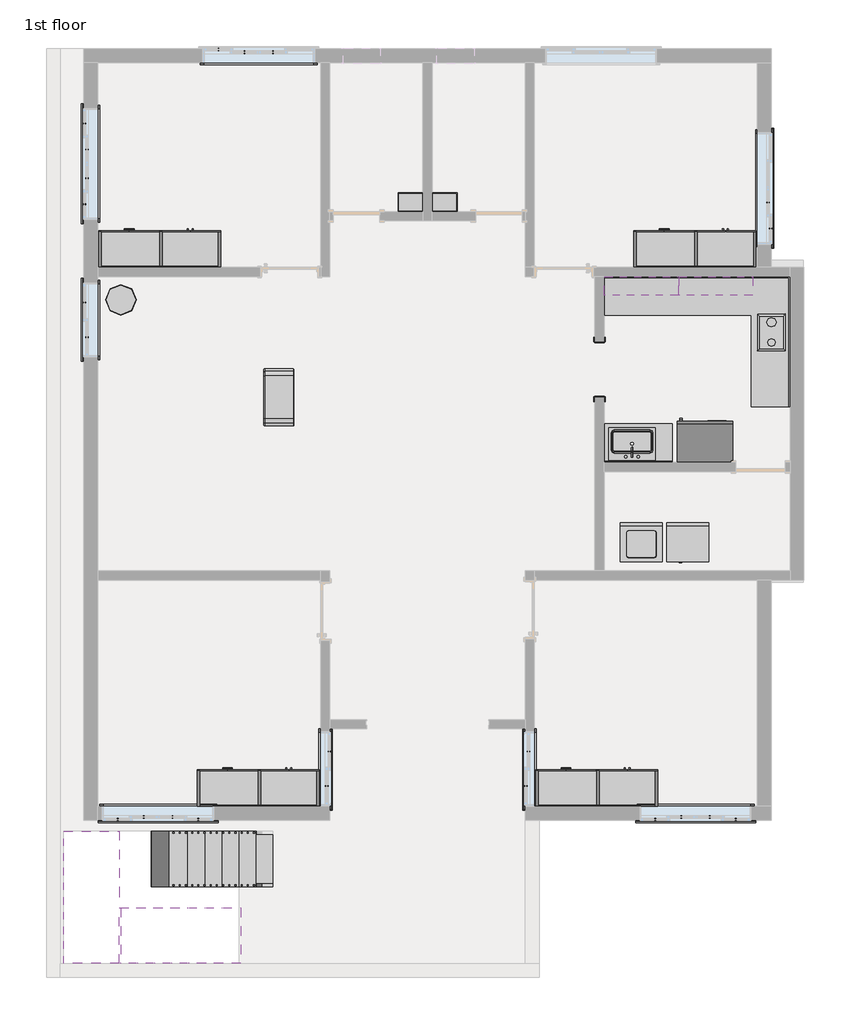
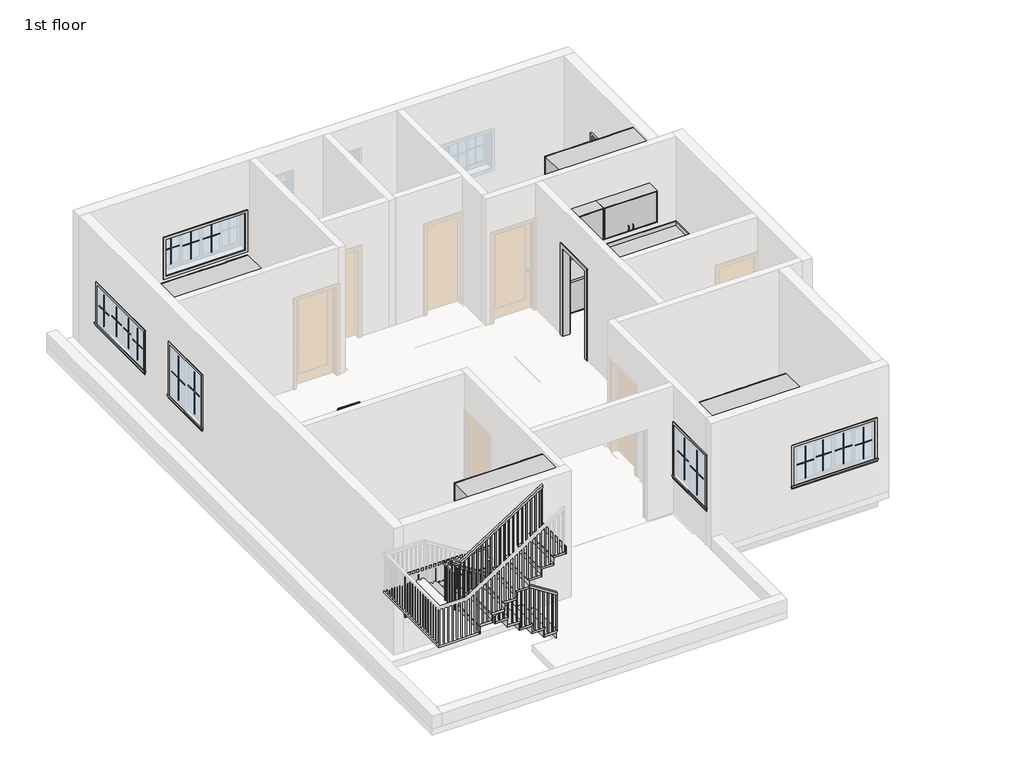
# One storey, part 3 of 4: 42 proxies, 15 furniture elements, 3 flow terminals, 2 stair flights, 1 railing, 1 slab.
# Revit data of these elements (continued)
# Elements 37, 38, 39, 40, 41 (IfcBuildingElementProxy, "Trim-Window-Interior-Flat : Picture Frame")
#   Opening Width = 6' - 0"
#   Opening Height = 3' - 0"
#   Trim Material = Wood - Stained
#   Phase Created = New Construction
#   Materials on its faces: "Wood - Stained"
# Element 42 (IfcBuildingElementProxy, "Washer : 27\" x 25\" x 35\"")
#   Phase Created = New Construction
#   Materials on its faces: "Metal - Paint Finish - Ivory,Matte"
# Element 43 (IfcFlowTerminal, "Sink - Work : 20\"x18\" 2")
#   Mark = "15"
#   Flow Pressure = 8.00 psi
#   Phase Created = New Construction
# Element 44 (IfcFlowTerminal, "Sink - Work : 20\"x18\" 2")
#   Mark = "16"
#   Flow Pressure = 8.00 psi
#   Phase Created = New Construction
# Element 45 (IfcFlowTerminal, "Sink Kitchen-Single : 30\" x 21\"")
#   Mark = "14"
#   Phase Created = New Construction
#   Materials on its faces: "Steel, Polished"
# Element 46 (IfcFurniture)
#   Phase Created = New Construction
# Element 47 (IfcFurniture)
#   Phase Created = New Construction
#   Materials on its faces: "Default", "Default 3", "Default 2"
# Elements 48, 49, 50, 51 (IfcFurniture, "1Wardrobe_6271 : 1Wardrobe_6271")
#   Phase Created = New Construction
#   Materials on its faces: "Phase - Demo", "Default Wall", "Phase - Exist", "Default"
# Element 52 (IfcFurniture, "48\" 2")
#   Phase Created = New Construction
#   Materials on its faces: "Cabinet", "Cabinets - Handles", "Cabinets"
# Element 53 (IfcFurniture, "48\" 3")
#   Phase Created = New Construction
#   Materials on its faces: "Cabinet", "Cabinets - Handles", "Cabinets"
# Element 54 (IfcFurniture, "Base Cabinet-Combo01 : 30\" 2")
#   Phase Created = New Construction
#   Materials on its faces: "Cabinet"
# Element 55 (IfcFurniture, "Base Cabinet-Corner Unit-Square : 36\"")
#   Phase Created = New Construction
#   Materials on its faces: "Cabinets", "Cabinets - Handles"
# Element 56 (IfcFurniture, "Counter Top w Sink Hole : 24\" Depth")
#   Sink Opening Width = 2' - 3"
#   Sink Opening Depth = 1' - 3"
#   Sink Location To Wall = 0' - 6"
#   Sink Location = 2' - 2"
#   Length = 3' - 8"
#   Phase Created = New Construction
#   Materials on its faces: "Counter Top"
# Element 57 (IfcFurniture, "Counter Top-L Shaped : 24\" Depth")
#   Length - Leg 2 = 10' - 0"
#   Length - Leg 1 = 7' - 0"
#   Phase Created = New Construction
#   Materials on its faces: "Counter Top"
# Element 58 (IfcFurniture, "Table-Trio End : 20\" Diameter")
#   Phase Created = New Construction
#   Materials on its faces: "Wood - Birch", "Laminate - Ivory,Matte"
# Elements 59, 60 (IfcFurniture, "Upper Cabinet-Pass-Thru : 48\" x 30\" x 12\"")
#   Phase Created = New Construction
#   Materials on its faces: "Cabinet"
# Element 61 (IfcRailing, "Handrail - Rectangular")
#   Phase Created = New Construction
# Element 62 (IfcSlab, "Non-Monolithic Landing")
#   Phase Created = New Construction
# Elements 63, 64 (IfcStairFlight, "2\" Tread 1\" Nosing 1/4\" Riser")
#   Phase Created = New Construction
# Materials
#   "Metal - Chrome": colour RGB 17 17 17, transparency 0
#   "Metal - Steel, Polished": colour RGB 57 57 57, transparency 0
#   "Metal - Paint Finish - Ivory,Glossy": colour RGB 247 247 239, transparency 0
#   "Door - Frame": colour RGB 118 70 51, transparency 0, Cost = 0
#   "Metal - Paint Finish - Ivory,Matte": colour RGB 247 247 239, transparency 0
#   "Steel, Polished": class "Metal", colour RGB 192 192 192, transparency 0, Description = "Polished steel", Cost = 0
#   "Cabinets - Handles": colour RGB 57 57 57, transparency 0
#   "Cabinets": colour RGB 249 249 249, transparency 0
#   "Wood - Birch": colour RGB 230 196 162, transparency 0
#   "Laminate - Ivory,Matte": colour RGB 127 127 127, transparency 0
#   "Clad - White": class "Wood", colour RGB 242 242 238, transparency 0, Cost = 0
#   "Wood - Stained": class "Wood", colour RGB 224 178 126, transparency 0, Cost = 0
#   "Default": colour RGB 127 127 127, transparency 0, Cost = 0
#   "Default 3": class "Glass", colour RGB 127 127 127, transparency 0
#   "Default 2": class "Plastic", colour RGB 127 127 127, transparency 0
#   "Phase - Demo": class "System", colour RGB 255 0 0, transparency 0.4, Cost = 0
#   "Default Wall": colour RGB 128 128 128, transparency 0, Cost = 0
#   "Phase - Exist": class "System", colour RGB 127 127 127, transparency 0, Cost = 0
#   "Cabinet": colour RGB 204 122 2, transparency 0
#   "Counter Top": class "Wood", colour RGB 226 177 128, transparency 0
